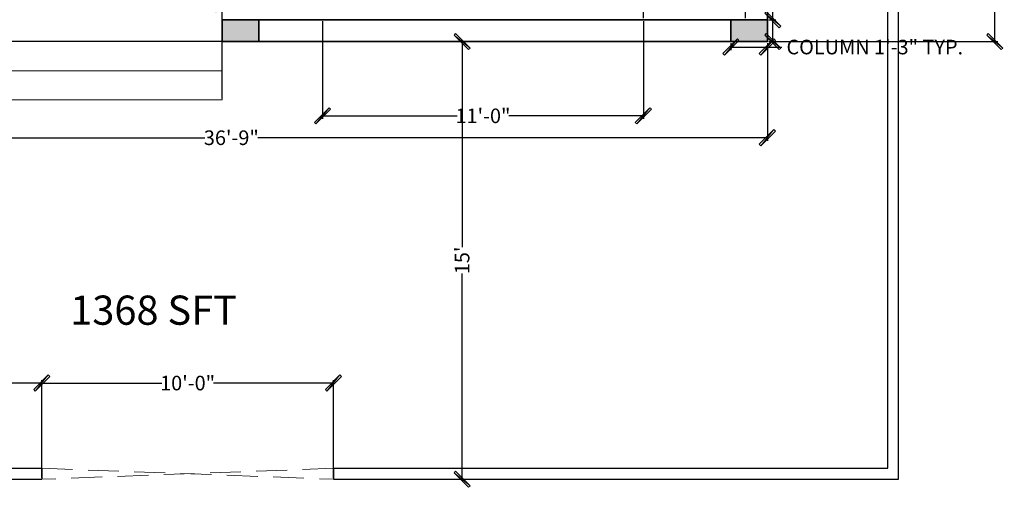
# Model space of a CAD drawing. Units: inches. Extents: x 1018 to 2596, y 723 to 1501.
# Tile 2 of 6: x 1276 to 1681, y 723 to 916. Entities that reach past the tile are written whole.
import ezdxf

# ---------------------------------------------------------------- set-up
doc = ezdxf.new("R2010")
doc.units = ezdxf.units.IN
doc.linetypes.add('DASHED', pattern=[19.05, 12.7, -6.35])
doc.layers.get('Defpoints').update_dxf_attribs({"lineweight": 0})
for name, color, linetype, lineweight in [('A-ANNO-DIMS', 2, 'Continuous', 13), ('A-AREA-IDEN', 7, 'Continuous', 18), ('A-COLS', 7, 'Continuous', 35), ('A-FLOR', 7, 'Continuous', 25), ('A-FLOR-STRS', 7, 'Continuous', 18), ('A-WALL', 7, 'Continuous', 35), ('C-PROP', 7, 'Continuous', 25), ('C-PROP-GATE', 7, 'DASHED', 13)]:
    doc.layers.add(name, color=color, linetype=linetype, lineweight=lineweight)
doc.styles.get("Standard").update_dxf_attribs({"font": 'arial.ttf'})
doc.dimstyles.new('saketh', dxfattribs={"dimtxt": 6, "dimasz": 6, "dimexe": 1.25, "dimexo": 0.625, "dimtad": 0, "dimdec": 1, "dimlunit": 4, "dimtxsty": 'Standard', "dimblk": 'ARCHTICK', "dimcen": 2.5, "dimclrd": 256, "dimclre": 1, "dimadec": 0, "dimazin": 0, "dimtfac": 1, "dimtdec": 1, "dimtmove": 0, "dimatfit": 3, "dimldrblk": 'ARCHTICK', "dimfxl": 1, "dimtolj": 1, "dimarcsym": 0})

# ---------------------------------------------------------------- blocks, each defined once
blk = doc.blocks.new('_ArchTick')
for p, q in [((0.447, 0.553), (-0.553, -0.447)), ((-0.447, -0.553), (0.553, 0.447)), ((0.553, 0.447), (0.447, 0.553)), ((-0.553, -0.447), (-0.447, -0.553))]:
    blk.add_line(p, q)
mesh = blk.add_polyface()
corners = [(-0.447, -0.553), (0.447, 0.553), (-0.553, -0.447), (0.553, 0.447)]
mesh.append_faces([[corners[k] for k in face] for face in [(0, 1, 2), (1, 0, 3)]], dxfattribs={"vtx0": -1})
blk = doc.blocks.new('*D53')
at = {"layer": 'A-ANNO-DIMS', "color": 0, "lineweight": -2, "transparency": 16777216}
for p, q in [((1417.36, 906.73), (1459.37, 906.73)), ((1458.12, 906.73), (1458.12, 822.16)), ((1458.12, 726.73), (1458.12, 811.29)), ((1417.36, 726.73), (1459.37, 726.73))]:
    blk.add_line(p, q, dxfattribs=at)
at = {"layer": 'Defpoints', "color": 0, "transparency": 16777216}
for p in [(1416.73, 906.73), (1416.73, 726.73), (1458.12, 726.73)]:
    blk.add_point(p, dxfattribs=at)
at = {"layer": 'A-ANNO-DIMS', "color": 0, "lineweight": -2, "transparency": 16777216, "xscale": 6, "yscale": 6, "zscale": 6}
for p, rotation in [((1458.12, 906.73), 90), ((1458.12, 726.73), 270)]:
    blk.add_blockref('_ArchTick', p, dxfattribs=dict(at, rotation=rotation))
at = {"layer": 'A-ANNO-DIMS', "color": 0, "transparency": 16777216, "insert": (1458.12, 816.73), "char_height": 6, "attachment_point": 5, "rotation": 90}
blk.add_mtext("\\A1;15'", dxfattribs=at)
blk = doc.blocks.new('COLUMN-15X9-IN')
h = blk.add_hatch(color=256)
h.dxf.hatch_style = 1
h.paths.add_polyline_path([(15, 0), (15, 9), (0, 9), (0, 0)])
blk.add_lwpolyline([(15, 9), (15, 0), (0, 0), (0, 9)], close=True)
blk = doc.blocks.new('*D57')
at = {"layer": 'A-ANNO-DIMS', "color": 1, "lineweight": -2, "transparency": 16777216}
for p, q in [((1568.69, 906.1), (1568.69, 903.23)), ((1583.69, 906.1), (1583.69, 903.23))]:
    blk.add_line(p, q, dxfattribs=at)
at = {"layer": 'A-ANNO-DIMS', "lineweight": -2, "transparency": 16777216}
for p, q in [((1568.69, 904.48), (1583.69, 904.48)), ((1583.69, 904.48), (1589.69, 904.48))]:
    blk.add_line(p, q, dxfattribs=at)
at = {"layer": 'Defpoints', "color": 0, "transparency": 16777216}
for p in [(1568.69, 906.73), (1583.69, 906.73), (1583.69, 904.48)]:
    blk.add_point(p, dxfattribs=at)
at = {"layer": 'A-ANNO-DIMS', "lineweight": -2, "transparency": 16777216, "xscale": 6, "yscale": 6, "zscale": 6, "rotation": 180}
blk.add_blockref('_ArchTick', (1568.69, 904.48), dxfattribs=at)
at = {"layer": 'A-ANNO-DIMS', "lineweight": -2, "transparency": 16777216, "xscale": 6, "yscale": 6, "zscale": 6}
blk.add_blockref('_ArchTick', (1583.69, 904.48), dxfattribs=at)
at = {"layer": 'A-ANNO-DIMS', "color": 0, "transparency": 16777216, "insert": (1627.89, 904.48), "char_height": 6, "attachment_point": 5}
blk.add_mtext('\\A1;COLUMN 1\'-3" TYP.', dxfattribs=at)
blk = doc.blocks.new('*D58')
at = {"layer": 'A-ANNO-DIMS', "lineweight": -2, "transparency": 16777216}
for p, q in [((1585.94, 915.73), (1585.94, 921.73)), ((1585.94, 906.73), (1585.94, 915.73))]:
    blk.add_line(p, q, dxfattribs=at)
at = {"layer": 'A-ANNO-DIMS', "color": 1, "lineweight": -2, "transparency": 16777216}
for p, q in [((1584.31, 915.73), (1587.19, 915.73)), ((1584.31, 906.73), (1587.19, 906.73))]:
    blk.add_line(p, q, dxfattribs=at)
at = {"layer": 'Defpoints', "color": 0, "transparency": 16777216}
for p in [(1583.69, 915.73), (1585.94, 915.73), (1583.69, 906.73)]:
    blk.add_point(p, dxfattribs=at)
at = {"layer": 'A-ANNO-DIMS', "lineweight": -2, "transparency": 16777216, "xscale": 6, "yscale": 6, "zscale": 6}
for p, rotation in [((1585.94, 915.73), 90), ((1585.94, 906.73), 270)]:
    blk.add_blockref('_ArchTick', p, dxfattribs=dict(at, rotation=rotation))
at = {"layer": 'A-ANNO-DIMS', "color": 0, "transparency": 16777216, "insert": (1585.94, 940.64), "char_height": 6, "attachment_point": 5, "rotation": 90}
blk.add_mtext('\\A1;0\'-9" TYP.', dxfattribs=at)
blk = doc.blocks.new('*D79')
at = {"layer": 'A-ANNO-DIMS', "color": 1, "lineweight": -2, "transparency": 16777216}
for p, q in [((1142.69, 906.1), (1142.69, 865.93)), ((1583.69, 906.1), (1583.69, 865.93))]:
    blk.add_line(p, q, dxfattribs=at)
at = {"layer": 'A-ANNO-DIMS', "lineweight": -2, "transparency": 16777216}
for p, q in [((1142.69, 867.18), (1352.26, 867.18)), ((1583.69, 867.18), (1374.12, 867.18))]:
    blk.add_line(p, q, dxfattribs=at)
at = {"layer": 'Defpoints', "color": 0, "transparency": 16777216}
for p in [(1142.69, 906.73), (1583.69, 906.73), (1142.69, 867.18)]:
    blk.add_point(p, dxfattribs=at)
at = {"layer": 'A-ANNO-DIMS', "lineweight": -2, "transparency": 16777216, "xscale": 6, "yscale": 6, "zscale": 6, "rotation": 180}
blk.add_blockref('_ArchTick', (1142.69, 867.18), dxfattribs=at)
at = {"layer": 'A-ANNO-DIMS', "lineweight": -2, "transparency": 16777216, "xscale": 6, "yscale": 6, "zscale": 6}
blk.add_blockref('_ArchTick', (1583.69, 867.18), dxfattribs=at)
at = {"layer": 'A-ANNO-DIMS', "color": 0, "transparency": 16777216, "insert": (1363.19, 867.18), "char_height": 6, "attachment_point": 5}
blk.add_mtext('\\A1;36\'-9"', dxfattribs=at)
blk = doc.blocks.new('*D81')
at = {"layer": 'A-ANNO-DIMS', "color": 1, "lineweight": -2, "transparency": 16777216}
for p, q in [((1584.31, 993.73), (1678.49, 993.73)), ((1584.31, 906.73), (1678.49, 906.73))]:
    blk.add_line(p, q, dxfattribs=at)
at = {"layer": 'A-ANNO-DIMS', "lineweight": -2, "transparency": 16777216}
for p, q in [((1677.24, 993.73), (1677.24, 958.8)), ((1677.24, 906.73), (1677.24, 941.65))]:
    blk.add_line(p, q, dxfattribs=at)
at = {"layer": 'Defpoints', "color": 0, "transparency": 16777216}
for p in [(1583.69, 993.73), (1677.24, 993.73), (1583.69, 906.73)]:
    blk.add_point(p, dxfattribs=at)
at = {"layer": 'A-ANNO-DIMS', "lineweight": -2, "transparency": 16777216, "xscale": 6, "yscale": 6, "zscale": 6}
for p, rotation in [((1677.24, 993.73), 90), ((1677.24, 906.73), 270)]:
    blk.add_blockref('_ArchTick', p, dxfattribs=dict(at, rotation=rotation))
at = {"layer": 'A-ANNO-DIMS', "color": 0, "transparency": 16777216, "insert": (1677.24, 950.23), "char_height": 6, "attachment_point": 5, "rotation": 90}
blk.add_mtext('\\A1;7\'-3"', dxfattribs=at)
blk = doc.blocks.new('*D82')
at = {"layer": 'A-ANNO-DIMS', "color": 1, "lineweight": -2, "transparency": 16777216}
for p, q in [((1052.69, 727.35), (1052.69, 767.53)), ((1285.19, 727.35), (1285.19, 767.53))]:
    blk.add_line(p, q, dxfattribs=at)
at = {"layer": 'A-ANNO-DIMS', "lineweight": -2, "transparency": 16777216}
for p, q in [((1052.69, 766.28), (1151.3, 766.28)), ((1285.19, 766.28), (1186.58, 766.28))]:
    blk.add_line(p, q, dxfattribs=at)
at = {"layer": 'Defpoints', "color": 0, "transparency": 16777216}
for p in [(1285.19, 766.28), (1052.69, 726.73), (1285.19, 726.73)]:
    blk.add_point(p, dxfattribs=at)
at = {"layer": 'A-ANNO-DIMS', "lineweight": -2, "transparency": 16777216, "xscale": 6, "yscale": 6, "zscale": 6, "rotation": 180}
blk.add_blockref('_ArchTick', (1052.69, 766.28), dxfattribs=at)
at = {"layer": 'A-ANNO-DIMS', "lineweight": -2, "transparency": 16777216, "xscale": 6, "yscale": 6, "zscale": 6}
blk.add_blockref('_ArchTick', (1285.19, 766.28), dxfattribs=at)
at = {"layer": 'A-ANNO-DIMS', "color": 0, "transparency": 16777216, "insert": (1168.94, 766.28), "char_height": 6, "attachment_point": 5}
blk.add_mtext('\\A1;19\'-4 1/2"', dxfattribs=at)
blk = doc.blocks.new('*D83')
at = {"layer": 'A-ANNO-DIMS', "color": 1, "lineweight": -2, "transparency": 16777216}
for p, q in [((1285.19, 727.35), (1285.19, 767.53)), ((1405.19, 727.35), (1405.19, 767.53))]:
    blk.add_line(p, q, dxfattribs=at)
at = {"layer": 'A-ANNO-DIMS', "lineweight": -2, "transparency": 16777216}
for p, q in [((1285.19, 766.28), (1334.54, 766.28)), ((1405.19, 766.28), (1355.84, 766.28))]:
    blk.add_line(p, q, dxfattribs=at)
at = {"layer": 'Defpoints', "color": 0, "transparency": 16777216}
for p in [(1405.19, 766.28), (1285.19, 726.73), (1405.19, 726.73)]:
    blk.add_point(p, dxfattribs=at)
at = {"layer": 'A-ANNO-DIMS', "lineweight": -2, "transparency": 16777216, "xscale": 6, "yscale": 6, "zscale": 6, "rotation": 180}
blk.add_blockref('_ArchTick', (1285.19, 766.28), dxfattribs=at)
at = {"layer": 'A-ANNO-DIMS', "lineweight": -2, "transparency": 16777216, "xscale": 6, "yscale": 6, "zscale": 6}
blk.add_blockref('_ArchTick', (1405.19, 766.28), dxfattribs=at)
at = {"layer": 'A-ANNO-DIMS', "color": 0, "transparency": 16777216, "insert": (1345.19, 766.28), "char_height": 6, "attachment_point": 5}
blk.add_mtext('\\A1;10\'-0"', dxfattribs=at)
blk = doc.blocks.new('*D84')
at = {"layer": 'A-ANNO-DIMS', "color": 1, "lineweight": -2, "transparency": 16777216}
for p, q in [((1157.69, 883.35), (1157.69, 923.53)), ((1359.46, 883.35), (1359.46, 923.53))]:
    blk.add_line(p, q, dxfattribs=at)
at = {"layer": 'A-ANNO-DIMS', "lineweight": -2, "transparency": 16777216}
for p, q in [((1157.69, 922.28), (1245.6, 922.28)), ((1359.46, 922.28), (1271.55, 922.28))]:
    blk.add_line(p, q, dxfattribs=at)
at = {"layer": 'Defpoints', "color": 0, "transparency": 16777216}
for p in [(1359.46, 922.28), (1157.69, 882.73), (1359.46, 882.73)]:
    blk.add_point(p, dxfattribs=at)
at = {"layer": 'A-ANNO-DIMS', "lineweight": -2, "transparency": 16777216, "xscale": 6, "yscale": 6, "zscale": 6, "rotation": 180}
blk.add_blockref('_ArchTick', (1157.69, 922.28), dxfattribs=at)
at = {"layer": 'A-ANNO-DIMS', "lineweight": -2, "transparency": 16777216, "xscale": 6, "yscale": 6, "zscale": 6}
blk.add_blockref('_ArchTick', (1359.46, 922.28), dxfattribs=at)
at = {"layer": 'A-ANNO-DIMS', "color": 0, "transparency": 16777216, "insert": (1258.57, 922.28), "char_height": 6, "attachment_point": 5}
blk.add_mtext('\\A1;16\'-10"', dxfattribs=at)
blk = doc.blocks.new('*D86')
at = {"layer": 'A-ANNO-DIMS', "color": 1, "lineweight": -2, "transparency": 16777216}
for p, q in [((1400.69, 915.1), (1400.69, 874.93)), ((1532.69, 915.1), (1532.69, 874.93))]:
    blk.add_line(p, q, dxfattribs=at)
at = {"layer": 'A-ANNO-DIMS', "lineweight": -2, "transparency": 16777216}
for p, q in [((1400.69, 876.18), (1456.04, 876.18)), ((1532.69, 876.18), (1477.34, 876.18))]:
    blk.add_line(p, q, dxfattribs=at)
at = {"layer": 'Defpoints', "color": 0, "transparency": 16777216}
for p in [(1400.69, 915.73), (1532.69, 915.73), (1400.69, 876.18)]:
    blk.add_point(p, dxfattribs=at)
at = {"layer": 'A-ANNO-DIMS', "lineweight": -2, "transparency": 16777216, "xscale": 6, "yscale": 6, "zscale": 6, "rotation": 180}
blk.add_blockref('_ArchTick', (1400.69, 876.18), dxfattribs=at)
at = {"layer": 'A-ANNO-DIMS', "lineweight": -2, "transparency": 16777216, "xscale": 6, "yscale": 6, "zscale": 6}
blk.add_blockref('_ArchTick', (1532.69, 876.18), dxfattribs=at)
at = {"layer": 'A-ANNO-DIMS', "color": 0, "transparency": 16777216, "insert": (1466.69, 876.18), "char_height": 6, "attachment_point": 5}
blk.add_mtext('\\A1;11\'-0"', dxfattribs=at)
blk = doc.blocks.new('*D87')
at = {"layer": 'A-ANNO-DIMS', "color": 1, "lineweight": -2, "transparency": 16777216}
for p, q in [((1532.69, 916.35), (1532.69, 956.53)), ((1574.69, 916.35), (1574.69, 956.53))]:
    blk.add_line(p, q, dxfattribs=at)
at = {"layer": 'A-ANNO-DIMS', "lineweight": -2, "transparency": 16777216}
for p, q in [((1532.69, 955.28), (1545.09, 955.28)), ((1574.69, 955.28), (1562.28, 955.28))]:
    blk.add_line(p, q, dxfattribs=at)
at = {"layer": 'Defpoints', "color": 0, "transparency": 16777216}
for p in [(1574.69, 955.28), (1532.69, 915.73), (1574.69, 915.73)]:
    blk.add_point(p, dxfattribs=at)
at = {"layer": 'A-ANNO-DIMS', "lineweight": -2, "transparency": 16777216, "xscale": 6, "yscale": 6, "zscale": 6, "rotation": 180}
blk.add_blockref('_ArchTick', (1532.69, 955.28), dxfattribs=at)
at = {"layer": 'A-ANNO-DIMS', "lineweight": -2, "transparency": 16777216, "xscale": 6, "yscale": 6, "zscale": 6}
blk.add_blockref('_ArchTick', (1574.69, 955.28), dxfattribs=at)
at = {"layer": 'A-ANNO-DIMS', "color": 0, "transparency": 16777216, "insert": (1553.69, 955.28), "char_height": 6, "attachment_point": 5}
blk.add_mtext('\\A1;3\'-6"', dxfattribs=at)

msp = doc.modelspace()

# ---------------------------------------------------------------- linework, layer by layer
at = {"layer": 'A-FLOR'}
msp.add_line((1374.46, 906.73), (1142.69, 906.73), dxfattribs=at)
at = {"layer": 'A-FLOR-STRS'}
for p, q in [((1359.46, 906.73), (1359.46, 882.73)), ((1359.46, 894.73), (1157.69, 894.73)), ((1359.46, 882.73), (1157.69, 882.73))]:
    msp.add_line(p, q, dxfattribs=at)
at = {"layer": 'A-WALL'}
for p, q in [((1583.69, 1233.73), (1583.69, 906.73)), ((1574.69, 915.73), (1374.46, 915.73)), ((1374.46, 915.73), (1374.46, 906.73)), ((1583.69, 906.73), (1374.46, 906.73))]:
    msp.add_line(p, q, dxfattribs=at)
at = {"layer": 'C-PROP'}
for p, q in [((1285.19, 731.23), (1285.19, 726.73)), ((1405.19, 731.23), (1405.19, 726.73))]:
    msp.add_line(p, q, dxfattribs=at)
for points in [[(1405.19, 726.73), (1637.69, 726.73), (1637.69, 1473.73), (1052.69, 1473.73), (1052.69, 726.73), (1285.19, 726.73)], [(1405.19, 731.23), (1633.19, 731.23), (1633.19, 1469.23), (1057.19, 1469.23), (1057.19, 731.23), (1285.19, 731.23)]]:
    msp.add_lwpolyline(points, dxfattribs=at)
at = {"layer": 'C-PROP-GATE'}
for p, q in [((1285.19, 731.23), (1405.19, 726.73)), ((1405.19, 731.23), (1285.19, 726.73))]:
    msp.add_line(p, q, dxfattribs=at)

# ---------------------------------------------------------------- block references
at = {"layer": 'A-COLS'}
for p in [(1359.46, 906.72), (1568.69, 906.72)]:
    msp.add_blockref('COLUMN-15X9-IN', p, dxfattribs=at)

# ---------------------------------------------------------------- texts
at = {"layer": 'A-AREA-IDEN', "insert": (1296.9, 802.26), "char_height": 9, "attachment_point": 1}
msp.add_mtext_dynamic_manual_height_columns('\\A1;{\\H1.33334x;1368 SFT\\P\\H0.5x;      }', width=78.1633, gutter_width=51.3, heights=[43.97], dxfattribs=at)

# ---------------------------------------------------------------- dimensions: what is measured, and where the dimension line sits
at = {"layer": 'A-ANNO-DIMS'}
for base, p1, p2, angle, override, picture, middle in [((1677.24, 993.73), (1583.69, 906.73), (1583.69, 993.73), 90, {"dimdec": 1, "dimlfac": 1, "dimrnd": 0, "dimzin": 1, "dimdsep": 46, "dimlunit": 4, "dimfrac": 2}, '*D81', (1677.24, 950.23)), ((1400.69, 876.18), (1532.69, 915.73), (1400.69, 915.73), 180, {"dimdec": 1, "dimlfac": 1, "dimrnd": 0, "dimzin": 1, "dimdsep": 46, "dimlunit": 4, "dimfrac": 2}, '*D86', (1466.69, 876.18)), ((1458.12, 726.73), (1416.73, 906.73), (1416.73, 726.73), 90, {"dimclrd": 0, "dimclre": 0, "dimclrt": 0}, '*D53', (1458.12, 816.73)), ((1142.69, 867.18), (1583.69, 906.73), (1142.69, 906.73), 180, {"dimdec": 1, "dimlfac": 1, "dimrnd": 0, "dimzin": 1, "dimdsep": 46, "dimlunit": 4, "dimfrac": 2}, '*D79', (1363.19, 867.18))]:
    dim = msp.add_linear_dim(base=base, p1=p1, p2=p2, angle=angle, dimstyle='saketh', override=override, dxfattribs=at)
    dim.commit()
    dim.dimension.update_dxf_attribs({"geometry": picture, "text_midpoint": middle})
for base, p1, p2, picture, middle in [((1574.69, 955.28), (1532.69, 915.73), (1574.69, 915.73), '*D87', (1553.69, 955.28)), ((1359.46, 922.28), (1157.69, 882.73), (1359.46, 882.73), '*D84', (1258.57, 922.28)), ((1285.19, 766.28), (1052.69, 726.73), (1285.19, 726.73), '*D82', (1168.94, 766.28)), ((1405.19, 766.28), (1285.19, 726.73), (1405.19, 726.73), '*D83', (1345.19, 766.28))]:
    dim = msp.add_linear_dim(base=base, p1=p1, p2=p2, dimstyle='saketh', override={"dimdec": 1, "dimlfac": 1, "dimrnd": 0, "dimzin": 1, "dimdsep": 46, "dimlunit": 4, "dimfrac": 2}, dxfattribs=at)
    dim.commit()
    dim.dimension.update_dxf_attribs({"geometry": picture, "text_midpoint": middle})
dim = msp.add_linear_dim(base=(1585.94, 915.73), p1=(1583.69, 906.73), p2=(1583.69, 915.73), angle=90, text='<> TYP.', dimstyle='saketh', override={"dimdec": 1, "dimlfac": 1, "dimrnd": 0, "dimzin": 1, "dimdsep": 46, "dimlunit": 4, "dimfrac": 2}, dxfattribs=at)
dim.commit()
dim.dimension.update_dxf_attribs({"geometry": '*D58', "text_midpoint": (1585.94, 940.64)})
dim = msp.add_linear_dim(base=(1583.69, 904.48), p1=(1568.69, 906.73), p2=(1583.69, 906.73), text='COLUMN <> TYP.', dimstyle='saketh', override={"dimdec": 1, "dimlfac": 1, "dimrnd": 0, "dimzin": 1, "dimdsep": 46, "dimlunit": 4, "dimfrac": 2}, dxfattribs=at)
dim.commit()
dim.dimension.update_dxf_attribs({"geometry": '*D57', "text_midpoint": (1627.89, 904.48)})

doc.saveas('drawing.dxf')
